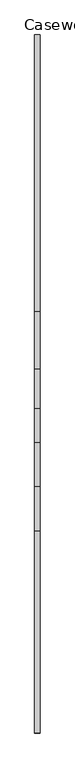
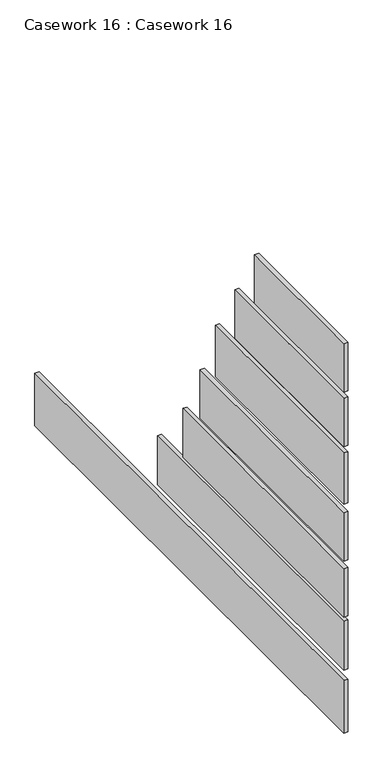
"""IFC4 building model written with IfcOpenShell, lengths in millimetres: furniture geometry, Casework 16 : Casework 16."""

from ifc_helpers import new_model, si_unit, frame, origin, place, context, project, spatial, polyline, outline, extrude, source, transform, mapped, element, save


def casework_16_casework_16_0ac3b185(model_context):
    return source(origin(), model_context, "Body", "SweptSolid", [
        extrude(outline(polyline([(14399.7923267, 6024.6064583), (14399.7923267, 5106.4593846), (14374.3923267, 5106.4593846), (14374.3923267, 6024.6064583), (14399.7923267, 6024.6064583)])), frame((0.0, 0.0, 3117.6699792), z_axis=(0.0, 0.0, 1.0), x_axis=(1.0, 0.0, 0.0)), (0.0, 0.0, 1.0), 304.8),
        extrude(outline(polyline([(14399.7923267, 6228.1496924), (14399.7923267, 5106.4593846), (14374.3923267, 5106.4593846), (14374.3923267, 6228.1496924), (14399.7923267, 6228.1496924)])), frame((0.0, 0.0, 2774.6394963), z_axis=(0.0, 0.0, 1.0), x_axis=(1.0, 0.0, 0.0)), (0.0, 0.0, 1.0), 304.8),
        extrude(outline(polyline([(14399.7923267, 6428.1746924), (14399.7923267, 5106.4593846), (14374.3923267, 5106.4593846), (14374.3923267, 6428.1746924), (14399.7923267, 6428.1746924)])), frame((0.0, 0.0, 2414.3803968), z_axis=(0.0, 0.0, 1.0), x_axis=(1.0, 0.0, 0.0)), (0.0, 0.0, 1.0), 322.0286166),
        extrude(outline(polyline([(14399.7923267, 6583.7496924), (14399.7923267, 5106.4593846), (14374.3923267, 5106.4593846), (14374.3923267, 6583.7496924), (14399.7923267, 6583.7496924)])), frame((0.0, 0.0, 2057.7422949), z_axis=(0.0, 0.0, 1.0), x_axis=(1.0, 0.0, 0.0)), (0.0, 0.0, 1.0), 304.8),
        extrude(outline(polyline([(14399.7923267, 6761.5496924), (14399.7923267, 5106.4593846), (14374.3923267, 5106.4593846), (14374.3923267, 6761.5496924), (14399.7923267, 6761.5496924)])), frame((0.0, 0.0, 1707.201272), z_axis=(0.0, 0.0, 1.0), x_axis=(1.0, 0.0, 0.0)), (0.0, 0.0, 1.0), 304.8),
        extrude(outline(polyline([(14399.7923267, 7024.4644217), (14399.7923267, 5106.4593846), (14374.3923267, 5106.4593846), (14374.3923267, 7024.4644217), (14399.7923267, 7024.4644217)])), frame((0.0, 0.0, 1374.4826326), z_axis=(0.0, 0.0, 1.0), x_axis=(1.0, 0.0, 0.0)), (0.0, 0.0, 1.0), 306.1010074),
        extrude(outline(polyline([(14399.7923267, 8284.2379112), (14399.7923267, 5106.4593846), (14374.3923267, 5106.4593846), (14374.3923267, 8284.2379112), (14399.7923267, 8284.2379112)])), frame((0.0, 0.0, 979.7962635), z_axis=(0.0, 0.0, 1.0), x_axis=(1.0, 0.0, 0.0)), (0.0, 0.0, 1.0), 330.2),
    ])


if __name__ == "__main__":
    model = new_model("IFC4")
    model_context = context("Model", 3, world=origin())
    ifc_project = project(units=[si_unit("LENGTHUNIT", "METRE", prefix="MILLI")], contexts=[model_context])
    site = spatial("IfcSite", under=ifc_project)
    building = spatial("IfcBuilding", under=site)
    placement = place(None, origin())
    casework_16_casework_16_shape = casework_16_casework_16_0ac3b185(model_context)
    element("IfcFurniture", 1, ObjectType="Casework 16 : Casework 16", at=placement, inside=building, context=model_context, shape_type="MappedRepresentation", body=[
        mapped(casework_16_casework_16_shape, transform((0.0, 0.0, 0.0), x_axis=(1.0, 0.0, 0.0), y_axis=(0.0, 1.0, 0.0), z_axis=(0.0, 0.0, 1.0))),
    ])
    save(model, "model.ifc")
